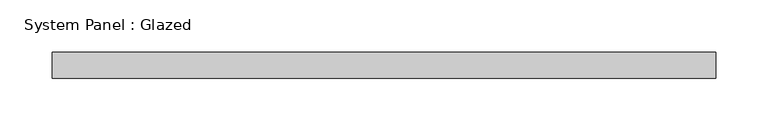
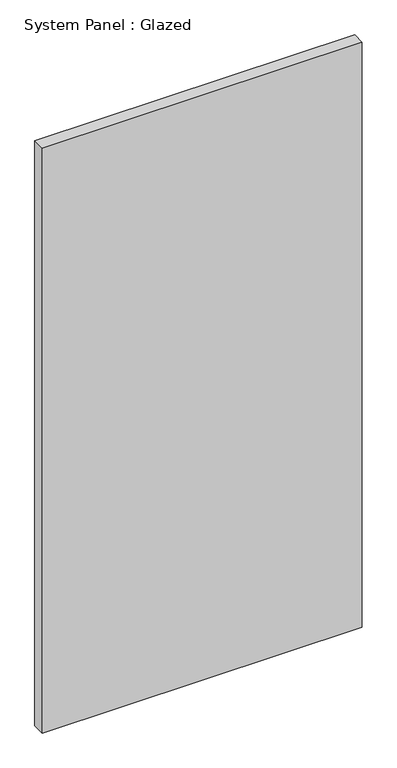
"""IFC4 building model written with IfcOpenShell, lengths in millimetres: plate geometry, System Panel : Glazed."""

from ifc_helpers import new_model, si_unit, origin, origin_with_axes, place, context, project, spatial, polyline, outline, extrude, source, transform, mapped, element, save


def system_panel_glazed_d508df5b(model_context):
    return source(origin(), model_context, "Body", "SweptSolid", [
        extrude(outline(polyline([(319.0875, 19.05), (-319.0875, 19.05), (-319.0875, 44.45), (319.0875, 44.45), (319.0875, 19.05)])), origin_with_axes(), (0.0, 0.0, 1.0), 1232.7734608),
    ])


if __name__ == "__main__":
    model = new_model("IFC4")
    model_context = context("Model", 3, world=origin())
    ifc_project = project(units=[si_unit("LENGTHUNIT", "METRE", prefix="MILLI")], contexts=[model_context])
    site = spatial("IfcSite", under=ifc_project)
    building = spatial("IfcBuilding", under=site)
    placement = place(None, origin())
    system_panel_glazed_shape = system_panel_glazed_d508df5b(model_context)
    element("IfcPlate", 1, ObjectType="System Panel : Glazed", at=placement, inside=building, context=model_context, shape_type="MappedRepresentation", body=[
        mapped(system_panel_glazed_shape, transform((0.0, 0.0, 0.0), x_axis=(1.0, 0.0, 0.0), y_axis=(0.0, 1.0, 0.0), z_axis=(0.0, 0.0, 1.0))),
    ])
    save(model, "model.ifc")

# Revit data of these elements
# Type "System Panel : Glazed"
#   Construction Type Id = "GSP4R"
#   Analytic Construction = "1/8 in Pilkington single glazing"
#   Visual Light Transmittance = 0.9
#   Solar Heat Gain Coefficient = 0.86
#   Heat Transfer Coefficient (U) = 1.18115 BTU/(h·ft²·°F)
#   Define Thermal Properties by = 1
# Element 1 (IfcPlate, "System Panel : Glazed")
#   Materials on its faces: "Glass"
# Materials
#   "Glass": class "Glass", colour RGB 0 128 192, transparency 0.75, Description = "Soda Lime Glass", Cost = 0
